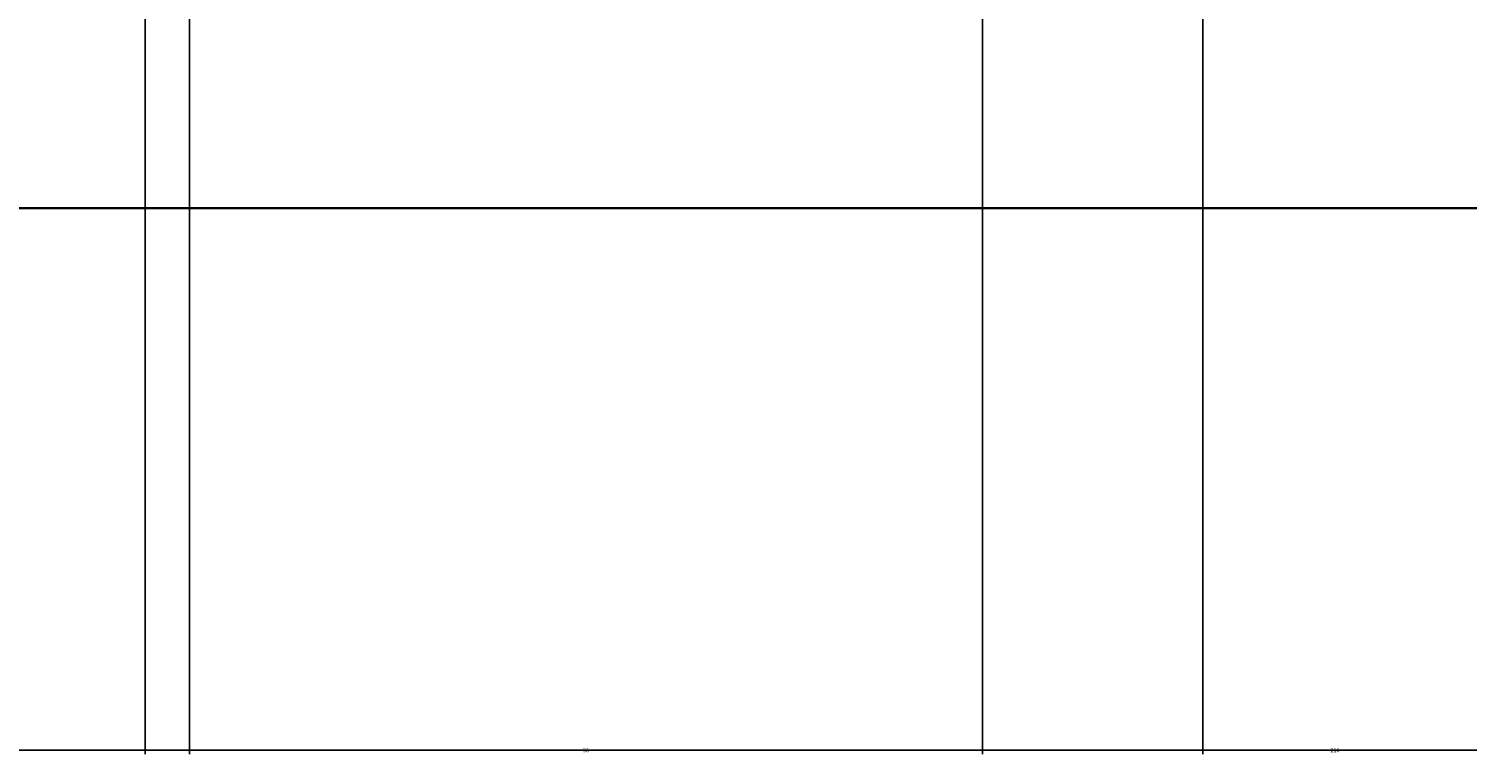
# Model space of a CAD drawing. Units: inches. Extents: x 8049 to 8459, y 820 to 1350.
# Tile 8 of 25: x 8132 to 8197, y 820 to 853. Entities that reach past the tile are written whole.
import ezdxf

# ---------------------------------------------------------------- set-up
doc = ezdxf.new("R2010")
doc.units = ezdxf.units.IN
doc.header["$MEASUREMENT"] = 0
doc.layers.add('A-ANNO-DIMS', color=2, linetype='Continuous', lineweight=18)
doc.layers.add('C-SITE-WALL', color=7, linetype='Continuous', lineweight=35)
doc.styles.get("Standard").update_dxf_attribs({"font": 'arial.ttf'})
doc.dimstyles.get("Standard").update_dxf_attribs({"dimtxt": 0.18, "dimasz": 0.18, "dimexe": 0.18, "dimexo": 0.0625, "dimgap": 0.09, "dimtad": 0, "dimtih": 1, "dimtoh": 1, "dimdec": 4, "dimzin": 0, "dimdsep": 46, "dimtxsty": 'Standard', "dimcen": 0.09, "dimadec": 0, "dimazin": 0, "dimtfac": 1, "dimtdec": 4, "dimtofl": 0, "dimtmove": 0, "dimatfit": 3, "dimfxl": 1, "dimtolj": 1, "dimtzin": 0, "dimarcsym": 0})

# ---------------------------------------------------------------- blocks, each defined once
blk = doc.blocks.new('*D58')
at = {"layer": 'A-ANNO-DIMS', "color": 0, "lineweight": -2, "transparency": 16777216}
for p, q in [((8139.397, 1162.808), (8139.397, 820.091)), ((8175.397, 1162.808), (8175.397, 820.091)), ((8139.577, 820.271), (8157.179, 820.271)), ((8175.217, 820.271), (8157.616, 820.271))]:
    blk.add_line(p, q, dxfattribs=at)
at = {"layer": 'A-ANNO-DIMS', "color": 0, "transparency": 16777216}
for points in [[(8139.577, 820.301), (8139.577, 820.241), (8139.397, 820.271)], [(8175.217, 820.301), (8175.217, 820.241), (8175.397, 820.271)]]:
    blk.add_solid(points, dxfattribs=at)
at = {"layer": 'Defpoints', "color": 0, "transparency": 16777216}
for p in [(8139.397, 1162.871), (8175.397, 1162.871), (8175.397, 820.271)]:
    blk.add_point(p, dxfattribs=at)
at = {"layer": 'A-ANNO-DIMS', "color": 0, "transparency": 16777216, "insert": (8157.397, 820.271), "char_height": 0.18, "attachment_point": 5}
blk.add_mtext('\\A1;36', dxfattribs=at)
blk = doc.blocks.new('*D70')
at = {"layer": 'A-ANNO-DIMS', "color": 0, "lineweight": -2, "transparency": 16777216}
for p, q in [((8083.397, 1045.808), (8083.397, 820.091)), ((8137.397, 1045.808), (8137.397, 820.091)), ((8083.577, 820.271), (8110.179, 820.271)), ((8137.217, 820.271), (8110.616, 820.271))]:
    blk.add_line(p, q, dxfattribs=at)
at = {"layer": 'A-ANNO-DIMS', "color": 0, "transparency": 16777216}
for points in [[(8083.577, 820.301), (8083.577, 820.241), (8083.397, 820.271)], [(8137.217, 820.301), (8137.217, 820.241), (8137.397, 820.271)]]:
    blk.add_solid(points, dxfattribs=at)
at = {"layer": 'Defpoints', "color": 0, "transparency": 16777216}
for p in [(8083.397, 1045.871), (8137.397, 1045.871), (8083.397, 820.271)]:
    blk.add_point(p, dxfattribs=at)
at = {"layer": 'A-ANNO-DIMS', "color": 0, "transparency": 16777216, "insert": (8110.397, 820.271), "char_height": 0.18, "attachment_point": 5}
blk.add_mtext('\\A1;54', dxfattribs=at)
blk = doc.blocks.new('*D71')
at = {"layer": 'A-ANNO-DIMS', "color": 0, "lineweight": -2, "transparency": 16777216}
for p, q in [((8185.397, 1045.808), (8185.397, 820.091)), ((8239.397, 1045.808), (8239.397, 820.091)), ((8185.577, 820.271), (8212.179, 820.271)), ((8239.217, 820.271), (8212.616, 820.271))]:
    blk.add_line(p, q, dxfattribs=at)
at = {"layer": 'A-ANNO-DIMS', "color": 0, "transparency": 16777216}
for points in [[(8185.577, 820.301), (8185.577, 820.241), (8185.397, 820.271)], [(8239.217, 820.301), (8239.217, 820.241), (8239.397, 820.271)]]:
    blk.add_solid(points, dxfattribs=at)
at = {"layer": 'Defpoints', "color": 0, "transparency": 16777216}
for p in [(8185.397, 1045.871), (8239.397, 1045.871), (8239.397, 820.271)]:
    blk.add_point(p, dxfattribs=at)
at = {"layer": 'A-ANNO-DIMS', "color": 0, "transparency": 16777216, "insert": (8212.397, 820.271), "char_height": 0.18, "attachment_point": 5}
blk.add_mtext('\\A1;54', dxfattribs=at)
blk = doc.blocks.new('*D76')
at = {"layer": 'A-ANNO-DIMS', "color": 0, "lineweight": -2, "transparency": 16777216}
for p, q in [((8083.397, 1054.808), (8083.397, 820.091)), ((8299.397, 1054.808), (8299.397, 820.091)), ((8083.577, 820.271), (8191.107, 820.271)), ((8299.217, 820.271), (8191.688, 820.271))]:
    blk.add_line(p, q, dxfattribs=at)
at = {"layer": 'A-ANNO-DIMS', "color": 0, "transparency": 16777216}
for points in [[(8083.577, 820.301), (8083.577, 820.241), (8083.397, 820.271)], [(8299.217, 820.301), (8299.217, 820.241), (8299.397, 820.271)]]:
    blk.add_solid(points, dxfattribs=at)
at = {"layer": 'Defpoints', "color": 0, "transparency": 16777216}
for p in [(8083.397, 1054.871), (8299.397, 1054.871), (8299.397, 820.271)]:
    blk.add_point(p, dxfattribs=at)
at = {"layer": 'A-ANNO-DIMS', "color": 0, "transparency": 16777216, "insert": (8191.397, 820.271), "char_height": 0.18, "attachment_point": 5}
blk.add_mtext('\\A1;216', dxfattribs=at)
blk = doc.blocks.new('*D88')
at = {"layer": 'A-ANNO-DIMS', "color": 0, "lineweight": -2, "transparency": 16777216}
for p, q in [((8083.397, 1162.808), (8083.397, 820.091)), ((8139.397, 1162.808), (8139.397, 820.091)), ((8083.577, 820.271), (8111.179, 820.271)), ((8139.217, 820.271), (8111.616, 820.271))]:
    blk.add_line(p, q, dxfattribs=at)
at = {"layer": 'A-ANNO-DIMS', "color": 0, "transparency": 16777216}
for points in [[(8083.577, 820.301), (8083.577, 820.241), (8083.397, 820.271)], [(8139.217, 820.301), (8139.217, 820.241), (8139.397, 820.271)]]:
    blk.add_solid(points, dxfattribs=at)
at = {"layer": 'Defpoints', "color": 0, "transparency": 16777216}
for p in [(8083.397, 1162.871), (8139.397, 1162.871), (8139.397, 820.271)]:
    blk.add_point(p, dxfattribs=at)
at = {"layer": 'A-ANNO-DIMS', "color": 0, "transparency": 16777216, "insert": (8111.397, 820.271), "char_height": 0.18, "attachment_point": 5}
blk.add_mtext('\\A1;56', dxfattribs=at)

msp = doc.modelspace()

# ---------------------------------------------------------------- linework, layer by layer
at = {"layer": 'C-SITE-WALL'}
msp.add_line((8074.3974, 844.8706), (8219.8974, 844.8706), dxfattribs=at)

# ---------------------------------------------------------------- dimensions: what is measured, and where the dimension line sits
at = {"layer": 'A-ANNO-DIMS'}
for base, p1, p2, picture, middle in [((8139.3974, 820.2706), (8083.3974, 1162.8706), (8139.3974, 1162.8706), '*D88', (8111.3974, 820.2706)), ((8175.3974, 820.2706), (8139.3974, 1162.8706), (8175.3974, 1162.8706), '*D58', (8157.3974, 820.2706)), ((8299.3974, 820.2706), (8083.3974, 1054.8706), (8299.3974, 1054.8706), '*D76', (8191.3974, 820.2706)), ((8083.3974, 820.2706), (8137.3974, 1045.8706), (8083.3974, 1045.8706), '*D70', (8110.3974, 820.2706)), ((8239.3974, 820.2706), (8185.3974, 1045.8706), (8239.3974, 1045.8706), '*D71', (8212.3974, 820.2706))]:
    dim = msp.add_linear_dim(base=base, p1=p1, p2=p2, dimstyle='Standard', override={"dimdec": 0, "dimlfac": 1, "dimrnd": 0, "dimzin": 0, "dimdsep": 46, "dimlunit": 2}, dxfattribs=at)
    dim.commit()
    dim.dimension.update_dxf_attribs({"geometry": picture, "text_midpoint": middle})

doc.saveas('drawing.dxf')
